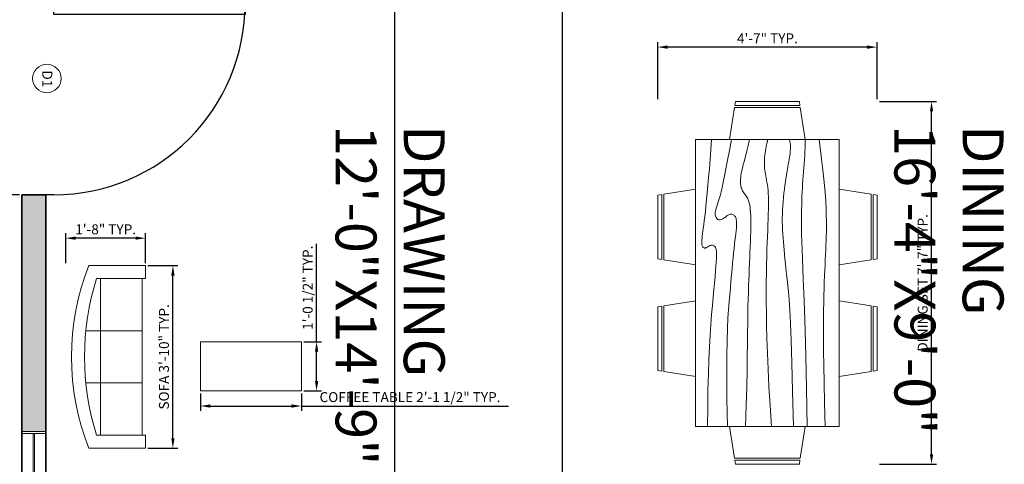
# Model space of a CAD drawing. Units: inches. Extents: x 7028582 to 7030319, y 63109697 to 63111305.
# Tile 15 of 18: x 7029748 to 7029995, y 63110742 to 63110853. Entities that reach past the tile are written whole.
import ezdxf

# ---------------------------------------------------------------- set-up
doc = ezdxf.new("R2010")
doc.units = ezdxf.units.IN
for name, color, linetype, lineweight in [('A-AREA-IDEN', 7, 'Continuous', 18), ('A-DOOR-IDEN', 20, 'Continuous', 13), ('A-WALL-PATT', 8, 'Continuous', 13), ('C-ANNO-DIMS', 7, 'Continuous', 18), ('doors', 20, 'Continuous', 25), ('furniture', 9, 'Continuous', 18), ('walls', 6, 'Continuous', 35), ('windows', 5, 'Continuous', 18)]:
    doc.layers.add(name, color=color, linetype=linetype, lineweight=lineweight)
doc.styles.get("Standard").update_dxf_attribs({"font": 'arial.ttf'})
doc.dimstyles.new('ISO-25', dxfattribs={"dimtxt": 2.5, "dimasz": 2.5, "dimexe": 1.25, "dimexo": 0.625, "dimtad": 1, "dimlunit": 4, "dimtxsty": 'Standard', "dimcen": 2.5, "dimadec": 0, "dimazin": 0, "dimtfac": 1, "dimtmove": 0, "dimatfit": 3, "dimfxl": 1, "dimarcsym": 0})

# ---------------------------------------------------------------- blocks, each defined once
blk = doc.blocks.new('*U2')
for p, q in [((0, 0), (0, -5)), ((30, 0), (30, -5))]:
    blk.add_line(p, q)
blk.add_lwpolyline([(0, 0), (0, 30), (1.75, 30), (1.75, 0)], close=True)
blk.add_arc((0, 0), 30, 0, 90)
blk = doc.blocks.new('Dining Set - 36 x 72 in.')
for p, q in [((-22, 27.5), (-22.1562, 26.50042)), ((-22, 27.5), (-6, 27.5)), ((-5.8437, 26.49966), (-6, 27.5)), ((6, 27.5), (5.8438, 26.50042)), ((6, 27.5), (22, 27.5)), ((22.1563, 26.49966), (22, 27.5)), ((-22.2343, 26.00059), (-23.4847, 17.99762)), ((-22.2304, 26), (-5.7608, 26)), ((-5.8416, 26.5), (-22.1534, 26.5)), ((-4.5152, 17.99762), (-5.7655, 25.99926)), ((5.7657, 26.00059), (4.5153, 17.99762)), ((5.7696, 26), (22.2392, 26)), ((22.1584, 26.5), (5.8466, 26.5)), ((23.4848, 17.99762), (22.2345, 25.99926)), ((36, 18), (-36, 18)), ((-36, 18), (-36, -18)), ((36, -18), (36, 18)), ((-45.5, 8), (-44.5004, 8.15617)), ((-45.5, 8), (-45.5, -8)), ((-44.5, -8.15843), (-44.5, 8.15338)), ((-44.0006, 8.23428), (-35.9976, 9.48474)), ((-44, 8.23041), (-44, -8.23915)), ((44.0006, 8.23428), (35.9976, 9.48474)), ((44, 8.23041), (44, -8.23915)), ((44.5, -8.15843), (44.5, 8.15338)), ((45.5, 8), (44.5005, 8.15617)), ((45.5, 8), (45.5, -8)), ((-44.4997, -8.15631), (-45.5, -8)), ((-35.9976, -9.48476), (-43.9993, -8.2345)), ((35.9976, -9.48476), (43.9993, -8.2345)), ((44.4997, -8.15631), (45.5, -8)), ((-36, -18), (36, -18)), ((-22.2343, -26.0006), (-23.4847, -17.99762)), ((-4.5152, -17.99762), (-5.7655, -25.99928)), ((5.7657, -26.0006), (4.5153, -17.99762)), ((23.4848, -17.99762), (22.2345, -25.99928)), ((-22.2304, -26), (-5.7608, -26)), ((-22, -27.5), (-22.1562, -26.50044)), ((-5.8416, -26.5), (-22.1534, -26.5)), ((-5.8437, -26.49967), (-6, -27.5)), ((5.7696, -26), (22.2392, -26)), ((6, -27.5), (5.8438, -26.50044)), ((22.1584, -26.5), (5.8466, -26.5)), ((22.1563, -26.49967), (22, -27.5)), ((-22, -27.5), (-6, -27.5)), ((6, -27.5), (22, -27.5))]:
    blk.add_line(p, q)
for points in [[(-36, 15), (-31.1772, 14.97754), (-26.8079, 14.91406), (-22.8538, 14.81543), (-19.276, 14.6875), (-16.0362, 14.53613), (-13.0957, 14.36718), (-10.4159, 14.18652), (-7.9583, 14), (-5.6904, 13.81315), (-3.6035, 13.63021), (-1.6954, 13.45508), (0.0365, 13.29166), (1.5945, 13.14388), (2.9811, 13.01562), (4.1988, 12.9108), (5.25, 12.83333), (6.1393, 12.78613), (6.8802, 12.76823), (7.4883, 12.77767), (7.9792, 12.8125), (8.3685, 12.87077), (8.6719, 12.95052), (8.9049, 13.0498), (9.0833, 13.16666), (9.2205, 13.29899), (9.3216, 13.44401), (9.3895, 13.59879), (9.4271, 13.76041), (9.4373, 13.92594), (9.4232, 14.09245), (9.3875, 14.257), (9.3333, 14.41666), (9.2638, 14.56917), (9.1836, 14.71484), (9.0975, 14.85465), (9.0104, 14.98958), (8.9272, 15.1206), (8.8529, 15.2487), (8.7922, 15.37483), (8.75, 15.5), (8.7305, 15.62467), (8.7344, 15.74739), (8.7617, 15.86621), (8.8125, 15.97916), (8.8867, 16.08431), (8.9844, 16.17968), (9.1055, 16.26334), (9.25, 16.33333), (9.4189, 16.38802), (9.6172, 16.42708), (9.8506, 16.45052), (10.125, 16.45833), (10.4463, 16.45052), (10.8203, 16.42708), (11.2529, 16.38802), (11.75, 16.33333), (12.3184, 16.26318), (12.9694, 16.17838), (13.7151, 16.07991), (14.5677, 15.96875), (15.5395, 15.84586), (16.6426, 15.71224), (17.8893, 15.56884), (19.2917, 15.41666), (20.859, 15.25667), (22.5879, 15.08984), (24.4721, 14.91715), (26.5052, 14.73958), (28.6809, 14.5581), (30.9929, 14.3737), (33.4347, 14.18733), (36, 14)], [(-36, 10), (-28.9766, 10.14274), (-23.1725, 10.20442), (-18.4241, 10.19775), (-14.5677, 10.13541), (-11.4399, 10.03011), (-8.877, 9.89453), (-6.7154, 9.74137), (-4.7917, 9.58333), (-2.9698, 9.43082), (-1.2246, 9.28515), (0.4415, 9.14534), (2.026, 9.01041), (3.5266, 8.87939), (4.9408, 8.7513), (6.266, 8.62516), (7.5, 8.5), (8.6411, 8.37549), (9.6914, 8.2539), (10.6538, 8.13818), (11.5312, 8.03125), (12.3267, 7.93603), (13.043, 7.85547), (13.6831, 7.79248), (14.25, 7.75), (14.7471, 7.7303), (15.1797, 7.73307), (15.5537, 7.75732), (15.875, 7.80208), (16.1494, 7.86637), (16.3828, 7.94922), (16.5811, 8.04964), (16.75, 8.16666), (16.8944, 8.29915), (17.0143, 8.44531), (17.1089, 8.60319), (17.1771, 8.77083), (17.218, 8.94629), (17.2305, 9.1276), (17.2137, 9.31282), (17.1667, 9.5), (17.0895, 9.6875), (16.987, 9.875), (16.8649, 10.0625), (16.7292, 10.25), (16.5856, 10.4375), (16.4401, 10.625), (16.2985, 10.8125), (16.1667, 11), (16.05, 11.18733), (15.9518, 11.3737), (15.8752, 11.5581), (15.8229, 11.73958), (15.798, 11.91715), (15.8034, 12.08984), (15.842, 12.25667), (15.9167, 12.41666), (16.0295, 12.56836), (16.1784, 12.70833), (16.3605, 12.83268), (16.5729, 12.9375), (16.8127, 13.01888), (17.0768, 13.07291), (17.3625, 13.0957), (17.6667, 13.08333), (17.9894, 13.03312), (18.3418, 12.94726), (18.7382, 12.82918), (19.1927, 12.68229), (19.7195, 12.51001), (20.3327, 12.31575), (21.0465, 12.10294), (21.875, 11.875), (22.8357, 11.63354), (23.959, 11.37304), (25.2786, 11.08618), (26.8282, 10.76562), (28.6414, 10.40405), (30.752, 9.99414), (33.1936, 9.52856), (36, 9)], [(-36, 5.5), (-30.7157, 5.3348), (-26.069, 5.20963), (-21.9946, 5.11767), (-18.4271, 5.05208), (-15.3009, 5.00602), (-12.5508, 4.97265), (-10.1112, 4.94515), (-7.9167, 4.91666), (-5.909, 4.88167), (-4.0586, 4.83984), (-2.3429, 4.79215), (-0.7396, 4.73958), (0.7739, 4.6831), (2.22, 4.6237), (3.6213, 4.56233), (5, 4.5), (6.373, 4.43782), (7.7344, 4.3776), (9.0723, 4.32129), (10.375, 4.27083), (11.6309, 4.22819), (12.8281, 4.19531), (13.9551, 4.17415), (15, 4.16666), (15.954, 4.17448), (16.819, 4.19791), (17.6001, 4.23698), (18.3021, 4.29166), (18.9299, 4.36198), (19.4883, 4.44791), (19.9823, 4.54948), (20.4167, 4.66666), (20.7969, 4.79899), (21.1302, 4.94401), (21.4245, 5.09879), (21.6875, 5.26041), (21.9271, 5.42594), (22.1511, 5.59245), (22.3672, 5.757), (22.5834, 5.91666), (22.8065, 6.06868), (23.0404, 6.21093), (23.2879, 6.34147), (23.5521, 6.45833), (23.8358, 6.55957), (24.142, 6.64323), (24.4735, 6.70735), (24.8334, 6.75), (25.2235, 6.76969), (25.642, 6.76692), (26.0858, 6.74267), (26.5521, 6.69791), (27.0379, 6.63362), (27.5404, 6.55078), (28.0565, 6.45036), (28.5834, 6.33333), (29.1242, 6.19987), (29.7071, 6.04687), (30.3661, 5.87044), (31.1354, 5.66666), (32.0493, 5.43164), (33.142, 5.16146), (34.4475, 4.85221), (36, 4.5)], [(-36, -1), (-30.7915, -0.6591), (-26.0195, -0.38216), (-21.6519, -0.16284), (-17.6563, 0.00521), (-14.0005, 0.12833), (-10.6523, 0.21289), (-7.5796, 0.26522), (-4.75, 0.29166), (-2.134, 0.29793), (0.2878, 0.28711), (2.5317, 0.26163), (4.6146, 0.22396), (6.5529, 0.17651), (8.3633, 0.12174), (10.0623, 0.06209), (11.6667, 0), (13.1899, -0.06201), (14.6341, -0.1211), (15.9982, -0.17432), (17.2813, -0.21875), (18.4823, -0.25147), (19.6003, -0.26953), (20.6343, -0.27002), (21.5834, -0.25), (22.4481, -0.20768), (23.2357, -0.14584), (23.9549, -0.06836), (24.6146, 0.02083), (25.2235, 0.11784), (25.7904, 0.21875), (26.3241, 0.31966), (26.8334, 0.41666), (27.3265, 0.50618), (27.8099, 0.58593), (28.2894, 0.65397), (28.7709, 0.70833), (29.2601, 0.74707), (29.763, 0.76823), (30.2855, 0.76985), (30.8334, 0.75), (31.4088, 0.70784), (31.9994, 0.64713), (32.589, 0.57275), (33.1615, 0.48958), (33.7008, 0.4025), (34.1908, 0.3164), (34.6153, 0.23616), (34.9584, 0.16666), (35.2099, 0.11165), (35.3848, 0.07031), (35.504, 0.04069), (35.5886, 0.02083), (35.6594, 0.00879), (35.7377, 0.0026), (35.8442, 0.00032), (36, 0)], [(-36, -6.5), (-27.1843, -6.31267), (-20.084, -6.1263), (-14.469, -5.9419), (-10.1094, -5.76042), (-6.7752, -5.58285), (-4.2363, -5.41016), (-2.2629, -5.24333), (-0.625, -5.08334), (0.8708, -4.93099), (2.2715, -4.78646), (3.5872, -4.64974), (4.8281, -4.52084), (6.0046, -4.39974), (7.127, -4.28646), (8.2053, -4.18099), (9.25, -4.08334), (10.2705, -3.99382), (11.2734, -3.91407), (12.2647, -3.84603), (13.25, -3.79167), (14.2354, -3.75293), (15.2266, -3.73177), (16.2295, -3.73015), (17.25, -3.75), (18.2912, -3.79248), (19.3451, -3.85547), (20.4009, -3.93604), (21.4479, -4.03125), (22.4754, -4.13819), (23.4727, -4.25391), (24.4289, -4.37549), (25.3334, -4.5), (26.1785, -4.62492), (26.9694, -4.74935), (27.7145, -4.87281), (28.4219, -4.99479), (29.1, -5.11483), (29.7572, -5.23242), (30.4016, -5.34709), (31.0417, -5.45834), (31.6837, -5.56437), (32.3262, -5.65821), (32.9658, -5.73153), (33.599, -5.77604), (34.2224, -5.78345), (34.8327, -5.74545), (35.4264, -5.65373), (36, -5.5)], [(-36, -10), (-26.4022, -9.81299), (-18.4675, -9.62891), (-11.9839, -9.45069), (-6.7396, -9.28125), (-2.5226, -9.12354), (0.8789, -8.98047), (3.6769, -8.85498), (6.0833, -8.75), (8.2767, -8.66765), (10.3021, -8.60677), (12.1712, -8.56543), (13.8958, -8.54167), (15.4876, -8.53353), (16.9583, -8.53907), (18.3197, -8.55632), (19.5834, -8.58334), (20.7616, -8.61841), (21.8685, -8.66081), (22.9188, -8.71004), (23.9271, -8.76563), (24.9081, -8.82707), (25.8763, -8.89388), (26.8465, -8.96558), (27.8334, -9.04167), (28.8474, -9.12118), (29.8828, -9.20117), (30.93, -9.27824), (31.9792, -9.34896), (33.0205, -9.40991), (34.0443, -9.45768), (35.0407, -9.48885), (36, -9.5)], [(-36, -14.5), (-30.0881, -14.33513), (-25.0332, -14.21224), (-20.7312, -14.12647), (-17.0781, -14.07292), (-13.97, -14.04671), (-11.3027, -14.04297), (-8.9724, -14.05681), (-6.875, -14.08334), (-4.9224, -14.11833), (-3.0905, -14.16016), (-1.3709, -14.20785), (0.2448, -14.26042), (1.7647, -14.3169), (3.1973, -14.3763), (4.5507, -14.43767), (5.8333, -14.5), (7.0554, -14.5621), (8.235, -14.62175), (9.3922, -14.67652), (10.5469, -14.72396), (11.7192, -14.76164), (12.929, -14.78711), (14.1965, -14.79794), (15.5417, -14.79167), (16.9933, -14.76424), (18.6152, -14.70508), (20.4804, -14.60197), (22.6615, -14.44271), (25.2312, -14.21509), (28.2624, -13.9069), (31.8277, -13.50594), (36, -13)]]:
    blk.add_lwpolyline(points)
blk = doc.blocks.new('Sofa - Roundback 7 ft.')
for p, q in [((-12.00002, -32.4421), (-12.00003, -6.5971)), ((11.99997, -32.4421), (11.99998, -6.5971)), ((-36.000027, -34), (-36.000027, -11.4696)), ((-35.999844, -13.3819), (35.9998, -13.3819)), ((35.99998, -34), (35.99998, -11.4696)), ((-36.000027, -32.4421), (35.99998, -32.4421))]:
    blk.add_line(p, q)
for points in [[(-36.000027, -34), (-42.000027, -34), (-42.000027, -8)], [(41.99998, -8), (41.99998, -34), (35.99998, -34)]]:
    blk.add_lwpolyline(points)
for centre, radius, start, end in [((0, -114.25), 114.25, 68.43141, 111.5686), ((-0.00001, -127.1968), 121.1968, 72.72033, 107.2797)]:
    blk.add_arc(centre, radius, start, end)
blk = doc.blocks.new('WIN-SASH-24')
for p, q in [((24.05, 6), (0, 6)), ((0.5, 6), (0.5, 0)), ((23.55, 0), (23.55, 6)), ((23.55, 3.2), (0.5, 3.2)), ((23.55, 2.8), (0.5, 2.8)), ((0, 0), (24.05, 0))]:
    blk.add_line(p, q)
blk = doc.blocks.new('TABLE-COFFEE-RECT')
blk.add_lwpolyline([(25.34, 12.34), (0, 12.34), (0, 0), (25.34, 0)], close=True)
blk = doc.blocks.new('TAG-D1-MT-R')
blk.add_circle((3.58, 3.58), 3.58)
at = {"insert": (4.93, 5.6), "char_height": 2.5, "attachment_point": 1, "rotation": 270}
blk.add_mtext_dynamic_manual_height_columns('D1', width=2.5021, gutter_width=12.5, heights=[0], dxfattribs=at)
blk = doc.blocks.new('*D57')
at = {"layer": 'C-ANNO-DIMS', "color": 0, "lineweight": -2, "transparency": 16777216}
for p, q in [((7029779.83, 63110791.79), (7029787.33, 63110791.79)), ((7029786.08, 63110748.46), (7029786.08, 63110789.29)), ((7029779.83, 63110745.96), (7029787.33, 63110745.96))]:
    blk.add_line(p, q, dxfattribs=at)
at = {"layer": 'C-ANNO-DIMS', "color": 0, "lineweight": 100, "transparency": 16777216}
for points in [[(7029785.66, 63110789.29), (7029786.5, 63110789.29), (7029786.08, 63110791.79)], [(7029785.66, 63110748.46), (7029786.5, 63110748.46), (7029786.08, 63110745.96)]]:
    blk.add_solid(points, dxfattribs=at)
at = {"layer": 'Defpoints', "color": 0, "lineweight": 100, "transparency": 16777216}
for p in [(7029779.21, 63110791.79), (7029786.08, 63110791.79), (7029779.21, 63110745.96)]:
    blk.add_point(p, dxfattribs=at)
at = {"layer": 'C-ANNO-DIMS', "color": 0, "transparency": 16777216, "insert": (7029784.16, 63110768.88), "char_height": 2.5, "attachment_point": 5, "rotation": 90}
blk.add_mtext('SOFA 3\'-10" TYP.', dxfattribs=at)
blk = doc.blocks.new('*D58')
at = {"layer": 'C-ANNO-DIMS', "color": 0, "lineweight": -2, "transparency": 16777216}
for p, q in [((7029759.2, 63110792.41), (7029759.2, 63110799.91)), ((7029776.71, 63110798.66), (7029761.7, 63110798.66)), ((7029779.21, 63110792.41), (7029779.21, 63110799.91))]:
    blk.add_line(p, q, dxfattribs=at)
at = {"layer": 'C-ANNO-DIMS', "color": 0, "lineweight": 100, "transparency": 16777216}
for points in [[(7029761.7, 63110799.08), (7029761.7, 63110798.25), (7029759.2, 63110798.66)], [(7029776.71, 63110799.08), (7029776.71, 63110798.25), (7029779.21, 63110798.66)]]:
    blk.add_solid(points, dxfattribs=at)
at = {"layer": 'Defpoints', "color": 0, "lineweight": 100, "transparency": 16777216}
for p in [(7029759.2, 63110798.66), (7029759.2, 63110791.79), (7029779.21, 63110791.79)]:
    blk.add_point(p, dxfattribs=at)
at = {"layer": 'C-ANNO-DIMS', "color": 0, "transparency": 16777216, "insert": (7029769.21, 63110800.56), "char_height": 2.5, "attachment_point": 5}
blk.add_mtext('1\'-8" TYP.', dxfattribs=at)
blk = doc.blocks.new('*D73')
at = {"layer": 'C-ANNO-DIMS', "color": 0, "lineweight": -2, "transparency": 16777216}
for p, q in [((7029792.97, 63110759.72), (7029792.97, 63110755.3)), ((7029818.31, 63110759.72), (7029818.31, 63110755.3)), ((7029795.47, 63110756.55), (7029815.81, 63110756.55)), ((7029818.31, 63110756.55), (7029870.27, 63110756.55))]:
    blk.add_line(p, q, dxfattribs=at)
at = {"layer": 'C-ANNO-DIMS', "color": 0, "lineweight": 100, "transparency": 16777216}
for points in [[(7029795.47, 63110756.96), (7029795.47, 63110756.13), (7029792.97, 63110756.55)], [(7029815.81, 63110756.96), (7029815.81, 63110756.13), (7029818.31, 63110756.55)]]:
    blk.add_solid(points, dxfattribs=at)
at = {"layer": 'Defpoints', "color": 0, "lineweight": 100, "transparency": 16777216}
for p in [(7029792.97, 63110760.35), (7029818.31, 63110760.35), (7029818.31, 63110756.55)]:
    blk.add_point(p, dxfattribs=at)
at = {"layer": 'C-ANNO-DIMS', "color": 0, "transparency": 16777216, "insert": (7029845.54, 63110758.46), "char_height": 2.5, "attachment_point": 5}
blk.add_mtext('COFFEE TABLE 2\'-1 1/2" TYP.', dxfattribs=at)
blk = doc.blocks.new('*D74')
at = {"layer": 'C-ANNO-DIMS', "color": 0, "lineweight": -2, "transparency": 16777216}
for p, q in [((7029822.11, 63110772.69), (7029822.11, 63110797.27)), ((7029818.94, 63110772.69), (7029823.36, 63110772.69)), ((7029822.11, 63110762.85), (7029822.11, 63110770.19)), ((7029818.94, 63110760.35), (7029823.36, 63110760.35))]:
    blk.add_line(p, q, dxfattribs=at)
at = {"layer": 'C-ANNO-DIMS', "color": 0, "lineweight": 100, "transparency": 16777216}
for points in [[(7029821.7, 63110770.19), (7029822.53, 63110770.19), (7029822.11, 63110772.69)], [(7029821.7, 63110762.85), (7029822.53, 63110762.85), (7029822.11, 63110760.35)]]:
    blk.add_solid(points, dxfattribs=at)
at = {"layer": 'Defpoints', "color": 0, "lineweight": 100, "transparency": 16777216}
for p in [(7029818.31, 63110772.69), (7029822.11, 63110772.69), (7029818.31, 63110760.35)]:
    blk.add_point(p, dxfattribs=at)
at = {"layer": 'C-ANNO-DIMS', "color": 0, "transparency": 16777216, "insert": (7029820.2, 63110786.23), "char_height": 2.5, "attachment_point": 5, "rotation": 90}
blk.add_mtext('1\'-0 1/2" TYP.', dxfattribs=at)
blk = doc.blocks.new('*D77')
at = {"layer": 'C-ANNO-DIMS', "color": 0, "lineweight": -2, "transparency": 16777216}
for p, q in [((7029963.29, 63110832.95), (7029977.56, 63110832.95)), ((7029976.31, 63110744.45), (7029976.31, 63110830.45)), ((7029963.29, 63110741.95), (7029977.56, 63110741.95))]:
    blk.add_line(p, q, dxfattribs=at)
at = {"layer": 'C-ANNO-DIMS', "color": 0, "lineweight": 100, "transparency": 16777216}
for points in [[(7029975.9, 63110830.45), (7029976.73, 63110830.45), (7029976.31, 63110832.95)], [(7029975.9, 63110744.45), (7029976.73, 63110744.45), (7029976.31, 63110741.95)]]:
    blk.add_solid(points, dxfattribs=at)
at = {"layer": 'Defpoints', "color": 0, "lineweight": 100, "transparency": 16777216}
for p in [(7029962.66, 63110832.95), (7029976.31, 63110832.95), (7029962.66, 63110741.95)]:
    blk.add_point(p, dxfattribs=at)
at = {"layer": 'C-ANNO-DIMS', "color": 0, "transparency": 16777216, "insert": (7029974.4, 63110787.45), "char_height": 2.5, "attachment_point": 5, "rotation": 90}
blk.add_mtext('DINING SET 7\'-7" TYP.', dxfattribs=at)
blk = doc.blocks.new('*D78')
at = {"layer": 'C-ANNO-DIMS', "color": 0, "lineweight": -2, "transparency": 16777216}
for p, q in [((7029907.66, 63110833.57), (7029907.66, 63110847.85)), ((7029962.66, 63110833.57), (7029962.66, 63110847.85)), ((7029960.16, 63110846.6), (7029910.16, 63110846.6))]:
    blk.add_line(p, q, dxfattribs=at)
at = {"layer": 'C-ANNO-DIMS', "color": 0, "lineweight": 100, "transparency": 16777216}
for points in [[(7029910.16, 63110847.01), (7029910.16, 63110846.18), (7029907.66, 63110846.6)], [(7029960.16, 63110847.01), (7029960.16, 63110846.18), (7029962.66, 63110846.6)]]:
    blk.add_solid(points, dxfattribs=at)
at = {"layer": 'Defpoints', "color": 0, "lineweight": 100, "transparency": 16777216}
for p in [(7029907.66, 63110846.6), (7029907.66, 63110832.95), (7029962.66, 63110832.95)]:
    blk.add_point(p, dxfattribs=at)
at = {"layer": 'C-ANNO-DIMS', "color": 0, "transparency": 16777216, "insert": (7029935.16, 63110848.47), "char_height": 2.5, "attachment_point": 5}
blk.add_mtext('4\'-7" TYP.', dxfattribs=at)
blk = doc.blocks.new('*D104')
at = {"layer": 'C-ANNO-DIMS', "color": 0, "lineweight": -2, "transparency": 16777216}
for p, q in [((7029747.58, 63110857.56), (7028586.23, 63110857.56)), ((7028587.48, 63110812.06), (7028587.48, 63110855.06)), ((7029747.58, 63110809.56), (7028586.23, 63110809.56))]:
    blk.add_line(p, q, dxfattribs=at)
at = {"layer": 'C-ANNO-DIMS', "color": 0, "lineweight": 100, "transparency": 16777216}
for points in [[(7028587.06, 63110855.06), (7028587.89, 63110855.06), (7028587.48, 63110857.56)], [(7028587.06, 63110812.06), (7028587.89, 63110812.06), (7028587.48, 63110809.56)]]:
    blk.add_solid(points, dxfattribs=at)
at = {"layer": 'Defpoints', "color": 0, "lineweight": 100, "transparency": 16777216}
for p in [(7028587.48, 63110857.56), (7029748.21, 63110857.56), (7029748.21, 63110809.56)]:
    blk.add_point(p, dxfattribs=at)
at = {"layer": 'C-ANNO-DIMS', "color": 0, "transparency": 16777216, "insert": (7028585.57, 63110833.56), "char_height": 2.5, "attachment_point": 5, "rotation": 90}
blk.add_mtext('4\'-0"', dxfattribs=at)
blk = doc.blocks.new('*D105')
at = {"layer": 'C-ANNO-DIMS', "color": 0, "lineweight": -2, "transparency": 16777216}
for p, q in [((7029841.68, 63110859.93), (7029841.68, 63109697.14)), ((7029883.68, 63110859.93), (7029883.68, 63109697.14)), ((7029844.18, 63109698.39), (7029881.18, 63109698.39))]:
    blk.add_line(p, q, dxfattribs=at)
at = {"layer": 'C-ANNO-DIMS', "color": 0, "lineweight": 100, "transparency": 16777216}
for points in [[(7029844.18, 63109698.8), (7029844.18, 63109697.97), (7029841.68, 63109698.39)], [(7029881.18, 63109698.8), (7029881.18, 63109697.97), (7029883.68, 63109698.39)]]:
    blk.add_solid(points, dxfattribs=at)
at = {"layer": 'Defpoints', "color": 0, "lineweight": 100, "transparency": 16777216}
for p in [(7029841.68, 63110860.56), (7029883.68, 63110860.56), (7029883.68, 63109698.39)]:
    blk.add_point(p, dxfattribs=at)
at = {"layer": 'C-ANNO-DIMS', "color": 0, "transparency": 16777216, "insert": (7029862.68, 63109700.29), "char_height": 2.5, "attachment_point": 5}
blk.add_mtext('3\'-6"', dxfattribs=at)
blk = doc.blocks.new('*D112')
at = {"layer": 'C-ANNO-DIMS', "color": 0, "lineweight": -2, "transparency": 16777216}
for p, q in [((7029747.58, 63111033.06), (7028586.23, 63111033.06)), ((7028587.48, 63111030.56), (7028587.48, 63110548.06)), ((7029747.58, 63110545.56), (7028586.23, 63110545.56))]:
    blk.add_line(p, q, dxfattribs=at)
at = {"layer": 'C-ANNO-DIMS', "color": 0, "lineweight": 100, "transparency": 16777216}
for points in [[(7028587.06, 63111030.56), (7028587.89, 63111030.56), (7028587.48, 63111033.06)], [(7028587.06, 63110548.06), (7028587.89, 63110548.06), (7028587.48, 63110545.56)]]:
    blk.add_solid(points, dxfattribs=at)
at = {"layer": 'Defpoints', "color": 0, "lineweight": 100, "transparency": 16777216}
for p in [(7029748.21, 63111033.06), (7028587.48, 63110545.56), (7029748.21, 63110545.56)]:
    blk.add_point(p, dxfattribs=at)
at = {"layer": 'C-ANNO-DIMS', "color": 0, "transparency": 16777216, "insert": (7028585.56, 63110789.31), "char_height": 2.5, "attachment_point": 5, "rotation": 90}
blk.add_mtext('40\'-7 1/2"', dxfattribs=at)

msp = doc.modelspace()

# ---------------------------------------------------------------- hatches: boundary and pattern name
at = {"layer": 'A-WALL-PATT'}
h = msp.add_hatch(color=256, dxfattribs=at)
h.dxf.hatch_style = 1
h.paths.add_polyline_path([(7029754.205, 63110809.557), (7029748.205, 63110809.557), (7029748.205, 63110750.186), (7029754.205, 63110750.186)])

# ---------------------------------------------------------------- linework, layer by layer
at = {"layer": 'walls'}
for p, q in [((7029748.205, 63110545.557), (7029748.205, 63110809.557)), ((7029748.205, 63110809.557), (7029754.205, 63110809.557)), ((7029754.205, 63110716.557), (7029754.205, 63110809.557))]:
    msp.add_line(p, q, dxfattribs=at)
at = {"layer": 'windows'}
msp.add_line((7029754.205, 63110750.186), (7029748.205, 63110750.186), dxfattribs=at)

# ---------------------------------------------------------------- block references
at = {"layer": 'A-DOOR-IDEN'}
msp.add_blockref('TAG-D1-MT-R', (7029750.898, 63110835.142), dxfattribs=at)
at = {"layer": 'doors', "xscale": 1.599999999999999, "yscale": 1.599999999999999, "zscale": 1.599999999999999, "rotation": 270}
msp.add_blockref('*U2', (7029756.205, 63110857.557), dxfattribs=at)
at = {"layer": 'furniture', "rotation": 90}
msp.add_blockref('Dining Set - 36 x 72 in.', (7029935.163, 63110787.448), dxfattribs=at)
at = {"layer": 'furniture', "xscale": 0.5455524879488546, "yscale": 0.5455524879488546, "zscale": 0.5455524879488546, "rotation": 90}
msp.add_blockref('Sofa - Roundback 7 ft.', (7029760.658, 63110768.875), dxfattribs=at)
at = {"layer": 'furniture'}
msp.add_blockref('TABLE-COFFEE-RECT', (7029792.974, 63110760.346), dxfattribs=at)
at = {"layer": 'windows', "rotation": 89.99999995093432}
msp.add_blockref('WIN-SASH-24', (7029754.205, 63110726.137), dxfattribs=at)

# ---------------------------------------------------------------- texts
at = {"layer": 'A-AREA-IDEN', "char_height": 10.26307, "attachment_point": 1, "rotation": 270}
for s, insert in [('DRAWING\\P12\'-0"X14\'-9"', (7029854.241, 63110827.03)), ('DINING\\P16\'-4"X9\'-0"', (7029994.376, 63110827.03))]:
    msp.add_mtext_dynamic_manual_height_columns(s, width=82.04322, gutter_width=51.315, heights=[0], dxfattribs=dict(at, insert=insert))

# ---------------------------------------------------------------- dimensions: what is measured, and where the dimension line sits
at = {"layer": 'C-ANNO-DIMS'}
for base, p1, p2, picture, middle in [((7028587.475, 63110545.557), (7029748.205, 63111033.057), (7029748.205, 63110545.557), '*D112', (7028585.558, 63110789.307)), ((7028587.475, 63110857.557), (7029748.205, 63110809.557), (7029748.205, 63110857.557), '*D104', (7028585.574, 63110833.557))]:
    dim = msp.add_linear_dim(base=base, p1=p1, p2=p2, angle=90, dimstyle='ISO-25', override={"dimdec": 1, "dimlfac": 1, "dimrnd": 0, "dimzin": 1, "dimdsep": 46, "dimlunit": 4, "dimfrac": 2}, dxfattribs=at)
    dim.commit()
    dim.dimension.update_dxf_attribs({"geometry": picture, "text_midpoint": middle})
dim = msp.add_linear_dim(base=(7029883.685, 63109698.385), p1=(7029841.685, 63110860.557), p2=(7029883.685, 63110860.557), dimstyle='ISO-25', override={"dimdec": 1, "dimlfac": 1, "dimrnd": 0, "dimzin": 1, "dimdsep": 46, "dimlunit": 4, "dimfrac": 2}, dxfattribs=at)
dim.commit()
dim.dimension.update_dxf_attribs({"geometry": '*D105', "text_midpoint": (7029862.685, 63109700.288)})
for base, p1, p2, angle, text, picture, middle in [((7029907.663, 63110846.598), (7029962.663, 63110832.948), (7029907.663, 63110832.948), 180, '<> TYP.', '*D78', (7029935.163, 63110848.474)), ((7029976.313, 63110832.948), (7029962.663, 63110741.948), (7029962.663, 63110832.948), 90, 'DINING SET <> TYP.', '*D77', (7029974.396, 63110787.448)), ((7029759.203, 63110798.663), (7029779.207, 63110791.789), (7029759.203, 63110791.789), 180, '<> TYP.', '*D58', (7029769.205, 63110800.564)), ((7029822.113, 63110772.691), (7029818.312, 63110760.346), (7029818.312, 63110772.691), 90, '<> TYP.', '*D74', (7029820.195, 63110786.23)), ((7029786.081, 63110791.789), (7029779.207, 63110745.962), (7029779.207, 63110791.789), 90, 'SOFA <> TYP.', '*D57', (7029784.162, 63110768.875))]:
    dim = msp.add_linear_dim(base=base, p1=p1, p2=p2, angle=angle, text=text, dimstyle='ISO-25', override={"dimdec": 1, "dimlfac": 1, "dimrnd": 0, "dimzin": 1, "dimdsep": 46, "dimlunit": 4, "dimfrac": 2}, dxfattribs=at)
    dim.commit()
    dim.dimension.update_dxf_attribs({"geometry": picture, "text_midpoint": middle})
dim = msp.add_linear_dim(base=(7029818.312, 63110756.546), p1=(7029792.974, 63110760.346), p2=(7029818.312, 63110760.346), text='COFFEE TABLE <> TYP.', dimstyle='ISO-25', override={"dimdec": 1, "dimlfac": 1, "dimrnd": 0, "dimzin": 1, "dimdsep": 46, "dimlunit": 4, "dimfrac": 2}, dxfattribs=at)
dim.commit()
dim.dimension.update_dxf_attribs({"geometry": '*D73', "text_midpoint": (7029845.54, 63110758.464)})

doc.saveas('drawing.dxf')
